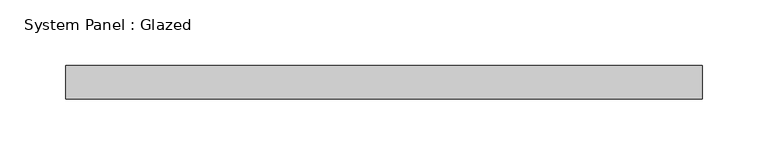
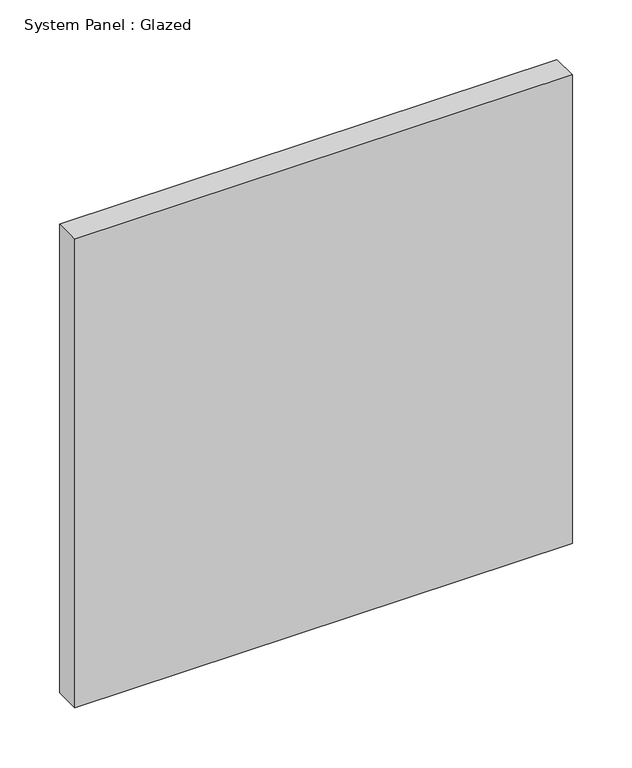
"""IFC4 building model written with IfcOpenShell, lengths in millimetres: plate geometry, System Panel : Glazed."""

from ifc_helpers import new_model, si_unit, origin, origin_with_axes, place, context, project, spatial, polyline, outline, extrude, source, transform, mapped, element, save


def system_panel_glazed_04707b35(model_context):
    return source(origin(), model_context, "Body", "SweptSolid", [
        extrude(outline(polyline([(241.3, 19.05), (-241.3, 19.05), (-241.3, 44.45), (241.3, 44.45), (241.3, 19.05)])), origin_with_axes(), (0.0, 0.0, 1.0), 480.6372143),
    ])


if __name__ == "__main__":
    model = new_model("IFC4")
    model_context = context("Model", 3, world=origin())
    ifc_project = project(units=[si_unit("LENGTHUNIT", "METRE", prefix="MILLI")], contexts=[model_context])
    site = spatial("IfcSite", under=ifc_project)
    building = spatial("IfcBuilding", under=site)
    placement = place(None, origin())
    system_panel_glazed_shape = system_panel_glazed_04707b35(model_context)
    element("IfcPlate", 1, ObjectType="System Panel : Glazed", at=placement, inside=building, context=model_context, shape_type="MappedRepresentation", body=[
        mapped(system_panel_glazed_shape, transform((0.0, 0.0, 0.0), x_axis=(1.0, 0.0, 0.0), y_axis=(0.0, 1.0, 0.0), z_axis=(0.0, 0.0, 1.0))),
    ])
    save(model, "model.ifc")

# Revit data of these elements
# Type "System Panel : Glazed"
#   Construction Type Id = "GSP4R"
#   Analytic Construction = "1/8 in Pilkington single glazing"
#   Visual Light Transmittance = 0.9
#   Solar Heat Gain Coefficient = 0.86
#   Heat Transfer Coefficient (U) = 1.18115 BTU/(h·ft²·°F)
#   Define Thermal Properties by = 1
# Element 1 (IfcPlate, "System Panel : Glazed")
#   Materials on its faces: "Glass"
# Materials
#   "Glass": class "Glass", colour RGB 0 128 192, transparency 0.75, Description = "Soda Lime Glass", Cost = 0
